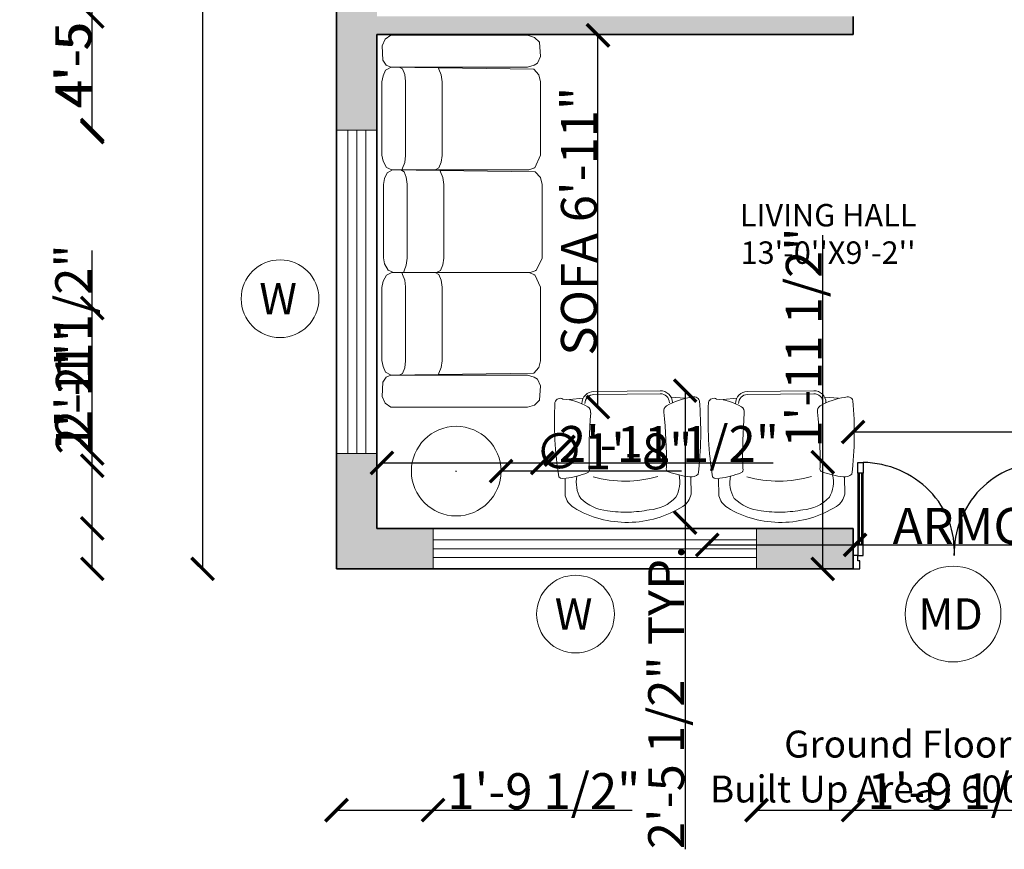
# Model space of a CAD drawing. Units: inches. Extents: x 2209 to 2954, y 1760 to 2265.
# Tile 1 of 7: x 2209 to 2428, y 1760 to 1945. Entities that reach past the tile are written whole.
import ezdxf

# ---------------------------------------------------------------- set-up
doc = ezdxf.new("R2010")
doc.units = ezdxf.units.IN
for name, color, linetype, lineweight in [('A-ANNO-DIMS', 2, 'Continuous', 18), ('A-ANNO-SYMB', 7, 'Continuous', 18), ('A-ANNO-TEXT', 7, 'Continuous', 25), ('A-AREA-IDEN', 7, 'Continuous', 18), ('A-FURN', 8, 'Continuous', 18), ('A-WALL-PATT', 30, 'Continuous', 13), ('DOOR', 240, 'Continuous', 25), ('WALL', 7, 'Continuous', 35), ('WINDOW', 190, 'Continuous', 18)]:
    doc.layers.add(name, color=color, linetype=linetype, lineweight=lineweight)
doc.layers.add('A-Glaz', color=92, linetype='Continuous')
doc.layers.add('MAIN DOOR', color=150, linetype='Continuous')
doc.styles.get("Standard").update_dxf_attribs({"font": 'arial.ttf'})
doc.dimstyles.get("Standard").update_dxf_attribs({"dimtxt": 8, "dimasz": 5, "dimexe": 0.18, "dimexo": 0.0625, "dimgap": 0.09, "dimtad": 1, "dimdec": 1, "dimzin": 0, "dimdsep": 46, "dimlunit": 4, "dimtxsty": 'Standard', "dimblk": 'ARCHTICK', "dimcen": 0.09, "dimse1": 1, "dimse2": 1, "dimadec": 0, "dimazin": 0, "dimtfac": 1, "dimtdec": 1, "dimtofl": 0, "dimtmove": 0, "dimatfit": 3, "dimfxl": 1, "dimtolj": 1, "dimtzin": 0, "dimarcsym": 0})

# ---------------------------------------------------------------- blocks, each defined once
blk = doc.blocks.new('A$C13CE0A17')
at = {"layer": 'A-Glaz'}
for p, q in [((0.01, 0.61), (0.01, 0.08)), ((0.03, 0.08), (0.03, 0.61))]:
    blk.add_line(p, q, dxfattribs=at)
blk.add_lwpolyline([(1.4, 0.08), (1.4, 0.61), (1.42, 0.61), (1.42, 0.08)], close=True, dxfattribs=at)
at = {"layer": 'MAIN DOOR'}
for p, q in [((0, 0.61), (0, 0.69)), ((0, 0.69), (0.04, 0.69)), ((0.04, 0.69), (0.04, 0.61)), ((0, 0.61), (0, 0.08)), ((0.04, 0.61), (0, 0.61)), ((0.04, 0.61), (0, 0.61)), ((0.03, 0.61), (0.01, 0.61)), ((0.04, 0.08), (0.04, 0.61)), ((0, 0.08), (0, 0)), ((0.04, 0.08), (0, 0.08)), ((0, 0.08), (0.04, 0.08)), ((0.01, 0.08), (0.03, 0.08)), ((0.04, 0), (0.04, 0.08)), ((-0.035, 0), (-0.035, -0.1)), ((0, 0), (-0.035, 0)), ((0, 0), (0.04, 0)), ((0, -0.04), (0, 0)), ((0.015, -0.04), (0, -0.04)), ((0.015, -0.05), (0.015, -0.04)), ((0.015, -0.1), (0.015, -0.05)), ((-0.035, -0.1), (0.015, -0.1))]:
    blk.add_line(p, q, dxfattribs=at)
for points in [[(1.39, 0.69), (1.39, 0.61), (1.43, 0.61), (1.43, 0.69)], [(1.39, 0.08), (1.39, 0.61), (1.43, 0.61), (1.43, 0.08)], [(1.39, 0), (1.39, 0.08), (1.43, 0.08), (1.43, 0)], [(1.43, 0), (1.465, 0), (1.465, -0.1), (1.415, -0.1), (1.415, -0.05), (1.415, -0.04), (1.43, -0.04)]]:
    blk.add_lwpolyline(points, close=True, dxfattribs=at)
blk.add_arc((1.3872, 0.017), 0.673, 89.76573, 181.44381, dxfattribs=at)
blk.add_ellipse((0.0389, 0.0511), major_axis=(0.6669, -0.1217), ratio=0.940794, start_param=0.11153, end_param=1.73917, dxfattribs=at)
blk = doc.blocks.new('12PCOU17')
at = {"color": 0, "linetype": 'ByBlock'}
for points in [[(-34.71, 34.72), (-33.66, 34.31), (-3.27, 34.3), (-1.81, 34.76), (-1.05, 35.2), (-0.38, 36.65), (-0.61, 39.84), (-1.73, 40.94), (-3.27, 41.4), (-33.66, 41.4), (-34.95, 40.5), (-35.65, 39.02), (-35.49, 35.83), (-34.71, 34.72)], [(-1.89, 11.91), (-1.66, 11.91), (-0.35, 14.68), (-0.35, 31.05), (-0.74, 32.58), (-1.89, 33.83), (-33.63, 34.3), (-34.84, 33.63), (-35.43, 32.38), (-35.68, 31), (-35.68, 14.74), (-35.43, 13.36), (-34.66, 11.99), (-33.44, 11.43), (-3, 11.44), (-1.66, 11.91)], [(-31.25, 11.43), (-31.06, 11.84), (-30.6, 13.09), (-30.4, 14.62), (-30.4, 31.12), (-30.6, 32.65), (-31.06, 33.9), (-31.81, 34.3)], [(-23.84, 11.43), (-22.99, 11.9), (-22.46, 13.15), (-22.23, 14.67), (-22.23, 31.07), (-22.46, 32.59), (-22.99, 33.84), (-23.12, 34.3)], [(-1.54, -10.96), (-1.31, -10.96), (0, -8.19), (0, 8.19), (-0.39, 9.71), (-1.54, 10.96), (-33.28, 11.44), (-34.5, 10.77), (-35.08, 9.51), (-35.33, 8.14), (-35.33, -8.13), (-35.08, -9.51), (-34.31, -10.87), (-33.1, -11.44), (-2.65, -11.43), (-1.31, -10.96)], [(-30.9, -11.44), (-30.72, -11.02), (-30.25, -9.77), (-30.05, -8.25), (-30.05, 8.26), (-30.25, 9.78), (-30.72, 11.03), (-31.47, 11.44)], [(-23.49, -11.44), (-22.64, -10.96), (-22.11, -9.72), (-21.88, -8.19), (-21.88, 8.2), (-22.11, 9.73), (-22.64, 10.97), (-22.77, 11.44)], [(-1.89, -11.91), (-1.66, -11.91), (-0.35, -14.68), (-0.35, -31.05), (-0.74, -32.58), (-1.89, -33.83), (-33.63, -34.3), (-34.84, -33.63), (-35.43, -32.38), (-35.68, -31), (-35.68, -14.74), (-35.43, -13.36), (-34.66, -11.99), (-33.44, -11.43), (-3, -11.44), (-1.66, -11.91)], [(-31.25, -11.43), (-31.06, -11.84), (-30.6, -13.09), (-30.4, -14.62), (-30.4, -31.12), (-30.6, -32.65), (-31.06, -33.9), (-31.81, -34.3)], [(-23.84, -11.43), (-22.99, -11.9), (-22.46, -13.15), (-22.23, -14.67), (-22.23, -31.07), (-22.46, -32.59), (-22.99, -33.84), (-23.12, -34.3)], [(-34.71, -34.72), (-33.66, -34.31), (-3.27, -34.3), (-1.81, -34.76), (-1.05, -35.2), (-0.38, -36.65), (-0.61, -39.84), (-1.73, -40.94), (-3.27, -41.4), (-33.66, -41.4), (-34.95, -40.5), (-35.65, -39.02), (-35.49, -35.83), (-34.71, -34.72)]]:
    blk.add_lwpolyline(points, dxfattribs=at)
blk = doc.blocks.new('A$C198557BC')
for p, q in [((-0.4117, 0.5807), (-0.4097, 0.6946)), ((0.4248, 0.5712), (0.4254, 0.6851)), ((-0.2994, 0.0834), (-0.2994, 0.0852)), ((0.3012, 0.0766), (0.3012, 0.0783)), ((-0.2905, 0.0459), (-0.3822, 0.0549)), ((0, 0), (-0.2203, 0.0025)), ((0.0002, 0.02), (-0.2201, 0.0225)), ((0, 0), (0.2203, -0.0025)), ((0.0002, 0.02), (0.2205, 0.0175)), ((0.2915, 0.0393), (0.3834, 0.0462))]:
    blk.add_line(p, q)
for centre, radius, start, end in [((-0.0029, 0.1962), 0.6755, 88.91413, 121.26982), ((0.0052, 0.1888), 0.6828, 57.60493, 89.60231), ((-0.1087, 0.5143), 0.2805, 94.11543, 135.13675), ((-0.0116, 0.1353), 0.6691, 87.97145, 100.08803), ((-0.0406, -0.2707), 1.076, 79.8996, 87.1923), ((0.1307, 0.5261), 0.2631, 42.84347, 86.21861), ((-0.2885, 0.6678), 0.1242, 121.56358, 167.53067), ((0.3036, 0.661), 0.1242, 11.16492, 57.13201), ((-0.132, 0.6064), 0.2049, 148.9368, 191.77668), ((0.1457, 0.6033), 0.2049, 346.91891, 29.75879), ((-0.0152, -0.1978), 0.7955, 73.93972, 105.23292), ((1.9871, 0.1943), 2.4688, 171.25046, 182.77379), ((-0.4204, 0.533), 0.0491, 69.35384, 131.44148), ((-0.4978, -0.067), 0.6529, 68.98758, 81.6584), ((-0.2691, 0.5224), 0.0208, 332.44605, 75.17429), ((0.2809, 0.5161), 0.0208, 103.52131, 206.24954), ((0.4962, -0.0783), 0.6529, 97.03719, 109.70801), ((0.4268, 0.5037), 0.0668, 46.11764, 99.16123), ((-1.9034, 0.2728), 2.3929, 354.99182, 6.69659), ((3.0866, 0.4124), 3.3387, 178.2785, 184.60096), ((-3.0764, 0.4826), 3.3387, 354.09463, 0.41709), ((-0.2813, 0.1392), 0.0403, 300.81783, 7.8066), ((0.2844, 0.1327), 0.0403, 170.889, 237.87776), ((-0.4437, 0.0838), 0.0362, 194.45648, 300.66989), ((-0.4522, 0.4253), 0.3736, 274.13358, 300.83861), ((-0.2194, 0.0825), 0.08, 179.3478, 269.3478), ((-0.2194, 0.0825), 0.06, 179.3478, 269.3478), ((0.2212, 0.0775), 0.08, 269.3478, 359.3478), ((0.2212, 0.0775), 0.06, 269.3478, 359.3478), ((0.4617, 0.4149), 0.3736, 237.85698, 264.56202), ((0.4455, 0.0737), 0.0362, 238.0257, 344.23911)]:
    blk.add_arc(centre, radius, start, end)
blk = doc.blocks.new('_ArchTick')
at = {"color": 0, "linetype": 'ByBlock', "const_width": 0.15}
blk.add_lwpolyline([(-0.5, -0.5), (0.5, 0.5)], dxfattribs=at)
blk = doc.blocks.new('*D14')
at = {"layer": 'A-ANNO-DIMS', "color": 0, "lineweight": -2, "transparency": 16777216}
blk.add_line((2249.34, 2182.29), (2249.34, 1822.29), dxfattribs=at)
at = {"layer": 'Defpoints', "color": 0, "transparency": 16777216}
for p in [(2279.15, 2182.29), (2249.34, 1822.29), (2279.15, 1822.29)]:
    blk.add_point(p, dxfattribs=at)
at = {"layer": 'A-ANNO-DIMS', "color": 0, "lineweight": -2, "transparency": 16777216, "xscale": 5, "yscale": 5, "zscale": 5}
for p, rotation in [((2249.34, 2182.29), 90), ((2249.34, 1822.29), 270)]:
    blk.add_blockref('_ArchTick', p, dxfattribs=dict(at, rotation=rotation))
at = {"layer": 'A-ANNO-DIMS', "color": 0, "transparency": 16777216, "insert": (2245.16, 2002.29), "char_height": 8, "attachment_point": 5, "rotation": 90}
blk.add_mtext("\\A1;30'", dxfattribs=at)
blk = doc.blocks.new('WIN-W-72IN')
for p, q in [((0, 6.5), (72, 6.5)), ((0, 4.5), (72, 4.5)), ((0, 2.5), (72, 2.5))]:
    blk.add_line(p, q)
blk.add_lwpolyline([(0, 9), (72, 9), (72, 0), (0, 0)], close=True)
blk = doc.blocks.new('TAG-OPENING-W')
blk.add_circle((0, 0), 8.66)
blk.add_text('W', height=7).set_placement((-4.62, -3.5))
blk = doc.blocks.new('*D49')
at = {"layer": 'A-ANNO-DIMS', "color": 0, "lineweight": -2, "transparency": 16777216}
for p, q in [((2394.15, 1852.78), (2439.18, 1852.78)), ((2439.18, 1852.78), (2532.94, 1852.78))]:
    blk.add_line(p, q, dxfattribs=at)
at = {"layer": 'Defpoints', "color": 0, "transparency": 16777216}
for p in [(2439.18, 1852.78), (2394.15, 1846.02), (2439.18, 1846.02)]:
    blk.add_point(p, dxfattribs=at)
at = {"layer": 'A-ANNO-DIMS', "color": 0, "lineweight": -2, "transparency": 16777216, "xscale": 5, "yscale": 5, "zscale": 5, "rotation": 180}
blk.add_blockref('_ArchTick', (2394.15, 1852.78), dxfattribs=at)
at = {"layer": 'A-ANNO-DIMS', "color": 0, "lineweight": -2, "transparency": 16777216, "xscale": 5, "yscale": 5, "zscale": 5}
blk.add_blockref('_ArchTick', (2439.18, 1852.78), dxfattribs=at)
at = {"layer": 'A-ANNO-DIMS', "color": 0, "transparency": 16777216, "insert": (2488.56, 1857.01), "char_height": 8, "attachment_point": 5}
blk.add_mtext('\\A1;MAIN DOOR 3\'-9"', dxfattribs=at)
blk = doc.blocks.new('*D50')
at = {"layer": 'A-ANNO-DIMS', "color": 0, "lineweight": -2, "transparency": 16777216}
for p, q in [((2387.4, 1846.02), (2387.4, 1896.57)), ((2387.4, 1822.29), (2387.4, 1846.02))]:
    blk.add_line(p, q, dxfattribs=at)
at = {"layer": 'Defpoints', "color": 0, "transparency": 16777216}
for p in [(2387.4, 1846.02), (2394.15, 1846.02), (2394.15, 1822.29)]:
    blk.add_point(p, dxfattribs=at)
at = {"layer": 'A-ANNO-DIMS', "color": 0, "lineweight": -2, "transparency": 16777216, "xscale": 5, "yscale": 5, "zscale": 5}
for p, rotation in [((2387.4, 1846.02), 90), ((2387.4, 1822.29), 270)]:
    blk.add_blockref('_ArchTick', p, dxfattribs=dict(at, rotation=rotation))
at = {"layer": 'A-ANNO-DIMS', "color": 0, "transparency": 16777216, "insert": (2383.17, 1873.8), "char_height": 8, "attachment_point": 5, "rotation": 90}
blk.add_mtext('\\A1;1\'-11 1/2"', dxfattribs=at)
blk = doc.blocks.new('*D59')
at = {"layer": 'A-ANNO-DIMS', "color": 0, "lineweight": -2, "transparency": 16777216}
for p, q in [((2361.69, 1827.63), (2394.59, 1827.63)), ((2394.59, 1827.63), (2511.71, 1827.63))]:
    blk.add_line(p, q, dxfattribs=at)
at = {"layer": 'Defpoints', "color": 0, "transparency": 16777216}
for p in [(2361.69, 1832.57), (2394.59, 1832.57), (2394.59, 1827.63)]:
    blk.add_point(p, dxfattribs=at)
at = {"layer": 'A-ANNO-DIMS', "color": 0, "lineweight": -2, "transparency": 16777216, "xscale": 5, "yscale": 5, "zscale": 5, "rotation": 180}
blk.add_blockref('_ArchTick', (2361.69, 1827.63), dxfattribs=at)
at = {"layer": 'A-ANNO-DIMS', "color": 0, "lineweight": -2, "transparency": 16777216, "xscale": 5, "yscale": 5, "zscale": 5}
blk.add_blockref('_ArchTick', (2394.59, 1827.63), dxfattribs=at)
at = {"layer": 'A-ANNO-DIMS', "color": 0, "transparency": 16777216, "insert": (2455.65, 1831.86), "char_height": 8, "attachment_point": 5}
blk.add_mtext('\\A1;ARMCHAIR 2\'-9" TYP.', dxfattribs=at)
blk = doc.blocks.new('*D60')
at = {"layer": 'A-ANNO-DIMS', "color": 0, "lineweight": -2, "transparency": 16777216}
for p, q in [((2356.76, 1861.96), (2356.76, 1832.57)), ((2356.76, 1832.57), (2356.76, 1759.85))]:
    blk.add_line(p, q, dxfattribs=at)
at = {"layer": 'Defpoints', "color": 0, "transparency": 16777216}
for p in [(2361.69, 1861.96), (2356.76, 1832.57), (2361.69, 1832.57)]:
    blk.add_point(p, dxfattribs=at)
at = {"layer": 'A-ANNO-DIMS', "color": 0, "lineweight": -2, "transparency": 16777216, "xscale": 5, "yscale": 5, "zscale": 5}
for p, rotation in [((2356.76, 1861.96), 90), ((2356.76, 1832.57), 270)]:
    blk.add_blockref('_ArchTick', p, dxfattribs=dict(at, rotation=rotation))
at = {"layer": 'A-ANNO-DIMS', "color": 0, "transparency": 16777216, "insert": (2352.53, 1793.71), "char_height": 8, "attachment_point": 5, "rotation": 90}
blk.add_mtext('\\A1;2\'-5 1/2" TYP.', dxfattribs=at)
blk = doc.blocks.new('*D63')
at = {"layer": 'A-ANNO-DIMS', "color": 0, "lineweight": -2, "transparency": 16777216}
blk.add_line((2337.35, 1858.3), (2337.35, 1941.1), dxfattribs=at)
at = {"layer": 'Defpoints', "color": 0, "transparency": 16777216}
for p in [(2324.93, 1941.1), (2337.35, 1941.1), (2324.93, 1858.3)]:
    blk.add_point(p, dxfattribs=at)
at = {"layer": 'A-ANNO-DIMS', "color": 0, "lineweight": -2, "transparency": 16777216, "xscale": 5, "yscale": 5, "zscale": 5}
for p, rotation in [((2337.35, 1941.1), 90), ((2337.35, 1858.3), 270)]:
    blk.add_blockref('_ArchTick', p, dxfattribs=dict(at, rotation=rotation))
at = {"layer": 'A-ANNO-DIMS', "color": 0, "transparency": 16777216, "insert": (2333.12, 1899.7), "char_height": 8, "attachment_point": 5, "rotation": 90}
blk.add_mtext('\\A1;SOFA 6\'-11"', dxfattribs=at)
blk = doc.blocks.new('*D64')
at = {"layer": 'A-ANNO-DIMS', "color": 0, "lineweight": -2, "transparency": 16777216}
for p, q in [((2289.25, 1845.88), (2324.93, 1845.88)), ((2324.93, 1845.88), (2376.37, 1845.88))]:
    blk.add_line(p, q, dxfattribs=at)
at = {"layer": 'Defpoints', "color": 0, "transparency": 16777216}
for p in [(2289.25, 1858.3), (2324.93, 1858.3), (2324.93, 1845.88)]:
    blk.add_point(p, dxfattribs=at)
at = {"layer": 'A-ANNO-DIMS', "color": 0, "lineweight": -2, "transparency": 16777216, "xscale": 5, "yscale": 5, "zscale": 5, "rotation": 180}
blk.add_blockref('_ArchTick', (2289.25, 1845.88), dxfattribs=at)
at = {"layer": 'A-ANNO-DIMS', "color": 0, "lineweight": -2, "transparency": 16777216, "xscale": 5, "yscale": 5, "zscale": 5}
blk.add_blockref('_ArchTick', (2324.93, 1845.88), dxfattribs=at)
at = {"layer": 'A-ANNO-DIMS', "color": 0, "transparency": 16777216, "insert": (2353.15, 1850.1), "char_height": 8, "attachment_point": 5}
blk.add_mtext('\\A1;2\'-11 1/2"', dxfattribs=at)
blk = doc.blocks.new('*D68')
at = {"layer": 'A-ANNO-DIMS', "color": 0, "lineweight": -2, "transparency": 16777216}
for p, q in [((2279.15, 1768.57), (2300.65, 1768.57)), ((2300.65, 1768.57), (2344.99, 1768.57))]:
    blk.add_line(p, q, dxfattribs=at)
at = {"layer": 'Defpoints', "color": 0, "transparency": 16777216}
for p in [(2279.15, 1822.29), (2300.65, 1822.29), (2300.65, 1768.57)]:
    blk.add_point(p, dxfattribs=at)
at = {"layer": 'A-ANNO-DIMS', "color": 0, "lineweight": -2, "transparency": 16777216, "xscale": 5, "yscale": 5, "zscale": 5, "rotation": 180}
blk.add_blockref('_ArchTick', (2279.15, 1768.57), dxfattribs=at)
at = {"layer": 'A-ANNO-DIMS', "color": 0, "lineweight": -2, "transparency": 16777216, "xscale": 5, "yscale": 5, "zscale": 5}
blk.add_blockref('_ArchTick', (2300.65, 1768.57), dxfattribs=at)
at = {"layer": 'A-ANNO-DIMS', "color": 0, "transparency": 16777216, "insert": (2325.32, 1772.79), "char_height": 8, "attachment_point": 5}
blk.add_mtext('\\A1;1\'-9 1/2"', dxfattribs=at)
blk = doc.blocks.new('*D69')
at = {"layer": 'A-ANNO-DIMS', "color": 0, "lineweight": -2, "transparency": 16777216}
for p, q in [((2372.65, 1768.57), (2394.15, 1768.57)), ((2394.15, 1768.57), (2438.49, 1768.57))]:
    blk.add_line(p, q, dxfattribs=at)
at = {"layer": 'Defpoints', "color": 0, "transparency": 16777216}
for p in [(2372.65, 1822.29), (2394.15, 1822.29), (2394.15, 1768.57)]:
    blk.add_point(p, dxfattribs=at)
at = {"layer": 'A-ANNO-DIMS', "color": 0, "lineweight": -2, "transparency": 16777216, "xscale": 5, "yscale": 5, "zscale": 5, "rotation": 180}
blk.add_blockref('_ArchTick', (2372.65, 1768.57), dxfattribs=at)
at = {"layer": 'A-ANNO-DIMS', "color": 0, "lineweight": -2, "transparency": 16777216, "xscale": 5, "yscale": 5, "zscale": 5}
blk.add_blockref('_ArchTick', (2394.15, 1768.57), dxfattribs=at)
at = {"layer": 'A-ANNO-DIMS', "color": 0, "transparency": 16777216, "insert": (2418.82, 1772.79), "char_height": 8, "attachment_point": 5}
blk.add_mtext('\\A1;1\'-9 1/2"', dxfattribs=at)
blk = doc.blocks.new('*D71')
at = {"layer": 'A-ANNO-DIMS', "color": 0, "lineweight": -2, "transparency": 16777216}
for p, q in [((2224.78, 1847.97), (2224.78, 1893.19)), ((2224.78, 1822.29), (2224.78, 1847.97))]:
    blk.add_line(p, q, dxfattribs=at)
at = {"layer": 'Defpoints', "color": 0, "transparency": 16777216}
for p in [(2224.78, 1847.97), (2279.15, 1847.97), (2279.15, 1822.29)]:
    blk.add_point(p, dxfattribs=at)
at = {"layer": 'A-ANNO-DIMS', "color": 0, "lineweight": -2, "transparency": 16777216, "xscale": 5, "yscale": 5, "zscale": 5}
for p, rotation in [((2224.78, 1847.97), 90), ((2224.78, 1822.29), 270)]:
    blk.add_blockref('_ArchTick', p, dxfattribs=dict(at, rotation=rotation))
at = {"layer": 'A-ANNO-DIMS', "color": 0, "transparency": 16777216, "insert": (2220.55, 1873.08), "char_height": 8, "attachment_point": 5, "rotation": 90}
blk.add_mtext('\\A1;2\'-1 1/2"', dxfattribs=at)
blk = doc.blocks.new('*D72')
at = {"layer": 'A-ANNO-DIMS', "color": 0, "lineweight": -2, "transparency": 16777216}
blk.add_line((2224.78, 1919.97), (2224.78, 1973.29), dxfattribs=at)
at = {"layer": 'Defpoints', "color": 0, "transparency": 16777216}
for p in [(2224.78, 1973.29), (2279.15, 1973.29), (2279.15, 1919.97)]:
    blk.add_point(p, dxfattribs=at)
at = {"layer": 'A-ANNO-DIMS', "color": 0, "lineweight": -2, "transparency": 16777216, "xscale": 5, "yscale": 5, "zscale": 5}
for p, rotation in [((2224.78, 1973.29), 90), ((2224.78, 1919.97), 270)]:
    blk.add_blockref('_ArchTick', p, dxfattribs=dict(at, rotation=rotation))
at = {"layer": 'A-ANNO-DIMS', "color": 0, "transparency": 16777216, "insert": (2220.55, 1946.63), "char_height": 8, "attachment_point": 5, "rotation": 90}
blk.add_mtext('\\A1;4\'-5 1/2"', dxfattribs=at)
blk = doc.blocks.new('*D78')
at = {"layer": 'A-ANNO-DIMS', "color": 0, "lineweight": -2, "transparency": 16777216}
blk.add_line((2224.78, 1945.29), (2224.78, 1981.29), dxfattribs=at)
at = {"layer": 'Defpoints', "color": 0, "transparency": 16777216}
for p in [(2224.78, 1981.29), (2288.15, 1981.29), (2288.15, 1945.29)]:
    blk.add_point(p, dxfattribs=at)
at = {"layer": 'A-ANNO-DIMS', "color": 0, "lineweight": -2, "transparency": 16777216, "xscale": 5, "yscale": 5, "zscale": 5}
for p, rotation in [((2224.78, 1981.29), 90), ((2224.78, 1945.29), 270)]:
    blk.add_blockref('_ArchTick', p, dxfattribs=dict(at, rotation=rotation))
at = {"layer": 'A-ANNO-DIMS', "color": 0, "transparency": 16777216, "insert": (2220.6, 1963.29), "char_height": 8, "attachment_point": 5, "rotation": 90}
blk.add_mtext('\\A1;3\'-0"', dxfattribs=at)
blk = doc.blocks.new('*D83')
at = {"layer": 'A-ANNO-DIMS', "color": 0, "lineweight": -2, "transparency": 16777216}
blk.add_line((2224.78, 1845.25), (2224.78, 1880.36), dxfattribs=at)
at = {"layer": 'Defpoints', "color": 0, "transparency": 16777216}
for p in [(2224.78, 1880.36), (2489.03, 1880.36), (2489.03, 1845.25)]:
    blk.add_point(p, dxfattribs=at)
at = {"layer": 'A-ANNO-DIMS', "color": 0, "lineweight": -2, "transparency": 16777216, "xscale": 5, "yscale": 5, "zscale": 5}
for p, rotation in [((2224.78, 1880.36), 90), ((2224.78, 1845.25), 270)]:
    blk.add_blockref('_ArchTick', p, dxfattribs=dict(at, rotation=rotation))
at = {"layer": 'A-ANNO-DIMS', "color": 0, "transparency": 16777216, "insert": (2220.67, 1862.81), "char_height": 8, "attachment_point": 5, "rotation": 90}
blk.add_mtext('\\A1;2\'-11"', dxfattribs=at)
blk = doc.blocks.new('*D84')
at = {"layer": 'A-ANNO-DIMS', "color": 0, "lineweight": -2, "transparency": 16777216}
for p, q in [((2224.78, 1845.25), (2224.78, 1870.94)), ((2224.78, 1831.29), (2224.78, 1845.25))]:
    blk.add_line(p, q, dxfattribs=at)
at = {"layer": 'Defpoints', "color": 0, "transparency": 16777216}
for p in [(2224.78, 1845.25), (2489.03, 1845.25), (2486.15, 1831.29)]:
    blk.add_point(p, dxfattribs=at)
at = {"layer": 'A-ANNO-DIMS', "color": 0, "lineweight": -2, "transparency": 16777216, "xscale": 5, "yscale": 5, "zscale": 5}
for p, rotation in [((2224.78, 1845.25), 90), ((2224.78, 1831.29), 270)]:
    blk.add_blockref('_ArchTick', p, dxfattribs=dict(at, rotation=rotation))
at = {"layer": 'A-ANNO-DIMS', "color": 0, "transparency": 16777216, "insert": (2220.67, 1860.6), "char_height": 8, "attachment_point": 5, "rotation": 90}
blk.add_mtext('\\A1;1\'-2"', dxfattribs=at)
blk = doc.blocks.new('*D88')
at = {"layer": 'A-ANNO-DIMS', "color": 0, "lineweight": -2, "transparency": 16777216}
blk.add_line((2224.78, 1919.53), (2224.78, 1973.14), dxfattribs=at)
at = {"layer": 'Defpoints', "color": 0, "transparency": 16777216}
for p in [(2224.78, 1973.14), (2629.22, 1973.14), (2629.22, 1919.53)]:
    blk.add_point(p, dxfattribs=at)
at = {"layer": 'A-ANNO-DIMS', "color": 0, "lineweight": -2, "transparency": 16777216, "xscale": 5, "yscale": 5, "zscale": 5}
for p, rotation in [((2224.78, 1973.14), 90), ((2224.78, 1919.53), 270)]:
    blk.add_blockref('_ArchTick', p, dxfattribs=dict(at, rotation=rotation))
at = {"layer": 'A-ANNO-DIMS', "color": 0, "transparency": 16777216, "insert": (2220.55, 1946.34), "char_height": 8, "attachment_point": 5, "rotation": 90}
blk.add_mtext('\\A1;4\'-5 1/2"', dxfattribs=at)
blk = doc.blocks.new('*D94')
at = {"layer": 'A-ANNO-DIMS', "color": 0, "lineweight": -2, "transparency": 16777216}
for p, q in [((2305.71, 1844.05), (2305.89, 1844.05)), ((2305.8, 1843.96), (2305.8, 1844.14)), ((2355.94, 1844.05), (2315.79, 1844.05))]:
    blk.add_line(p, q, dxfattribs=at)
at = {"layer": 'Defpoints', "color": 0, "transparency": 16777216}
for p in [(2295.82, 1844.05), (2315.79, 1844.05)]:
    blk.add_point(p, dxfattribs=at)
at = {"layer": 'A-ANNO-DIMS', "color": 0, "lineweight": -2, "transparency": 16777216, "xscale": 5, "yscale": 5, "zscale": 5, "rotation": 179.9972683628424}
blk.add_blockref('_ArchTick', (2315.79, 1844.05), dxfattribs=at)
at = {"layer": 'A-ANNO-DIMS', "color": 0, "transparency": 16777216, "insert": (2340.86, 1848.45), "char_height": 8, "attachment_point": 5, "rotation": 359.9973}
blk.add_mtext('\\A1;∅1\'-8"', dxfattribs=at)

msp = doc.modelspace()

# ---------------------------------------------------------------- hatches: boundary and pattern name
at = {"layer": 'A-WALL-PATT', "transparency": 33554585}
h = msp.add_hatch(color=256, dxfattribs=at)
h.dxf.hatch_style = 1
h.paths.add_polyline_path([(2519.15, 2182.29), (2402.15, 2182.29), (2402.15, 2173.29), (2444.15, 2173.29), (2444.15, 2154.12), (2448.15, 2154.12), (2448.15, 2173.29), (2510.15, 2173.29), (2510.15, 2167.29), (2519.15, 2167.29)])
h.paths.add_polyline_path([(2330.15, 2182.29), (2279.15, 2182.29), (2279.15, 2145.83), (2288.15, 2145.83), (2288.15, 2158.01), (2288.15, 2173.29), (2330.15, 2173.29)])
h.paths.add_polyline_path([(2288.15, 2073.83), (2279.15, 2073.83), (2279.15, 2009.29), (2288.15, 2009.29), (2288.15, 2037.29), (2404.15, 2037.29), (2404.15, 2041.29), (2288.15, 2041.29)])
h.paths.add_polyline_path([(2519.15, 2131.29), (2510.15, 2131.29), (2510.15, 2125.29), (2444.15, 2125.29), (2444.15, 2041.29), (2439.11, 2041.29), (2439.11, 2037.29), (2448.15, 2037.29), (2448.15, 2069.29), (2481.65, 2069.29), (2481.65, 2073.29), (2448.15, 2073.29), (2448.15, 2121.29), (2468.19, 2121.29), (2468.19, 2121.32), (2488.37, 2121.32), (2510.15, 2121.29), (2510.15, 2113.63), (2519.15, 2113.63)])
h.paths.add_polyline_path([(2519.15, 2077.63), (2510.15, 2077.63), (2510.15, 2073.32), (2510.17, 2073.32), (2510.15, 2069.19), (2510.15, 2043.25), (2519.15, 2043.25)], flags=17)
h.paths.add_polyline_path([(2519.15, 1971.25), (2510.15, 1971.25), (2510.15, 1945.29), (2444.15, 1945.29), (2444.15, 1937.21), (2448.15, 1937.21), (2448.15, 1941.29), (2510.15, 1941.29), (2510.15, 1922.29), (2519.15, 1922.29)])
h.paths.add_polyline_path([(2288.15, 1941.29), (2394.15, 1941.29), (2394.15, 1945.29), (2288.15, 1945.29), (2288.15, 1973.29), (2279.15, 1973.29), (2279.15, 1919.97), (2288.15, 1919.97)])
h.paths.add_polyline_path([(2300.65, 1831.29), (2288.15, 1831.29), (2288.15, 1847.97), (2279.15, 1847.97), (2279.15, 1822.29), (2300.65, 1822.29)])
h.paths.add_polyline_path([(2394.15, 1825.29), (2394.15, 1831.29), (2372.65, 1831.29), (2372.65, 1822.29), (2394.15, 1822.29)])
h.paths.add_polyline_path([(2449.17, 1831.29), (2448.15, 1831.29), (2448.15, 1899.32), (2444.15, 1899.32), (2444.15, 1831.29), (2439.18, 1831.29), (2439.18, 1822.29), (2449.17, 1822.29)])
h.paths.add_polyline_path([(2519.15, 1850.29), (2510.15, 1850.29), (2510.15, 1831.29), (2509.17, 1831.29), (2509.17, 1822.29), (2519.15, 1822.29)])
h.paths.add_polyline_path([(2638.22, 1941.29), (2744.22, 1941.29), (2744.22, 1945.29), (2638.22, 1945.29), (2638.22, 1973.14), (2629.22, 1973.14), (2629.22, 1919.53), (2638.22, 1919.53)])
h.paths.add_polyline_path([(2638.22, 1847.53), (2629.22, 1847.53), (2629.22, 1822.29), (2650.72, 1822.29), (2650.72, 1831.29), (2638.22, 1831.29)])
h.paths.add_polyline_path([(2638.22, 2037.29), (2754.22, 2037.29), (2754.22, 2041.29), (2638.22, 2041.29), (2638.22, 2074.27), (2629.22, 2074.27), (2629.22, 2009.14), (2638.22, 2009.14)])
h.paths.add_polyline_path([(2803.22, 1936.29), (2812.78, 1936.29), (2812.78, 1945.29), (2791.22, 1945.29), (2791.22, 1936.29), (2794.22, 1936.29), (2794.22, 1831.29), (2722.72, 1831.29), (2722.72, 1822.29), (2803.22, 1822.29)])
h.paths.add_polyline_path([(2869.22, 1955.43), (2860.22, 1955.43), (2860.22, 1945.29), (2853.36, 1945.29), (2853.36, 1936.29), (2869.22, 1936.29)])
h.paths.add_polyline_path([(2680.22, 2182.29), (2629.22, 2182.29), (2629.22, 2146.27), (2638.22, 2146.27), (2638.22, 2173.29), (2680.22, 2173.29)])
h.paths.add_polyline_path([(2869.22, 2182.29), (2752.22, 2182.29), (2752.22, 2173.29), (2794.22, 2173.29), (2794.22, 2142.92), (2798.22, 2142.92), (2798.22, 2173.29), (2860.22, 2173.29), (2860.22, 2158.46), (2869.22, 2158.46)])
h.paths.add_polyline_path([(2869.22, 2122.46), (2860.22, 2122.46), (2860.22, 2090.29), (2869.22, 2090.29)])

# ---------------------------------------------------------------- linework, layer by layer
at = {"layer": 'A-ANNO-SYMB'}
msp.add_circle((2416.4, 1812.24), 10.67, dxfattribs=at)
at = {"layer": 'A-FURN'}
msp.add_circle((2305.8, 1844.05), 9.98, dxfattribs=at)
at = {"layer": 'WALL'}
for p, q in [((2279.15, 2182.29), (2279.15, 1822.29)), ((2394.15, 1945.29), (2394.15, 1941.29)), ((2288.15, 1941.29), (2394.15, 1941.29)), ((2288.15, 1941.29), (2288.15, 1831.29)), ((2288.15, 1831.29), (2394.15, 1831.29)), ((2394.15, 1831.29), (2394.15, 1822.29)), ((2279.15, 1822.29), (2394.15, 1822.29))]:
    msp.add_line(p, q, dxfattribs=at)

# ---------------------------------------------------------------- block references
at = {"layer": 'A-ANNO-SYMB'}
for p in [(2266.58, 1882.44), (2332.36, 1812.22)]:
    msp.add_blockref('TAG-OPENING-W', p, dxfattribs=at)
at = {"layer": 'A-FURN'}
msp.add_blockref('12PCOU17', (2324.93, 1899.7), dxfattribs=at)
at = {"layer": 'A-FURN', "xscale": -33.52556732039916, "yscale": 33.52556732039916, "zscale": 33.52556732039916, "rotation": 180}
for p in [(2343.82, 1861.87), (2378.01, 1861.87)]:
    msp.add_blockref('A$C198557BC', p, dxfattribs=at)
at = {"layer": 'DOOR', "xscale": 30.0188950098318, "yscale": 30.0188950098318, "zscale": 30.0188950098318}
msp.add_blockref('A$C13CE0A17', (2395.21, 1825.29), dxfattribs=at)
at = {"layer": 'WINDOW', "rotation": 89.99999999999972}
msp.add_blockref('WIN-W-72IN', (2288.15, 1847.97), dxfattribs=at)
at = {"layer": 'WINDOW'}
msp.add_blockref('WIN-W-72IN', (2300.65, 1822.29), dxfattribs=at)

# ---------------------------------------------------------------- texts
at = {"layer": 'A-ANNO-SYMB'}
msp.add_text('MD', height=7, dxfattribs=at).set_placement((2408.69, 1808.74))
at = {"layer": 'A-ANNO-TEXT', "insert": (2338.03, 1786.28), "char_height": 6, "attachment_point": 1}
msp.add_mtext_dynamic_manual_height_columns('\\pxqc;Ground Floor Plan\\PBuilt Up Area : 600.00 Sq. ft', width=151.0778, gutter_width=102.73, heights=[0], dxfattribs=at)
at = {"layer": 'A-AREA-IDEN', "insert": (2366.02, 1903.54), "char_height": 5, "attachment_point": 1}
msp.add_mtext_dynamic_manual_height_columns("\\pxqc;LIVING HALL\\P13'-0''X9'-2''", width=45.1409, gutter_width=12.5, heights=[0], dxfattribs=at)

# ---------------------------------------------------------------- dimensions: what is measured, and where the dimension line sits
at = {"layer": 'A-ANNO-DIMS'}
for base, p1, p2, override, picture, middle in [((2249.34, 1822.29), (2279.15, 2182.29), (2279.15, 1822.29), {"dimclrd": 0, "dimclre": 0, "dimclrt": 0}, '*D14', (2245.16, 2002.29)), ((2224.78, 1981.29), (2288.15, 1945.29), (2288.15, 1981.29), {"dimdec": 1, "dimlfac": 1, "dimrnd": 0, "dimzin": 1, "dimdsep": 46, "dimlunit": 4, "dimfrac": 2}, '*D78', (2220.6, 1963.29)), ((2224.78, 1973.29), (2279.15, 1919.97), (2279.15, 1973.29), {"dimdec": 1, "dimlfac": 1, "dimrnd": 0, "dimzin": 1, "dimdsep": 46, "dimlunit": 4, "dimfrac": 2}, '*D72', (2220.55, 1946.63)), ((2224.78, 1973.14), (2629.22, 1919.53), (2629.22, 1973.14), {"dimdec": 1, "dimlfac": 1, "dimrnd": 0, "dimzin": 1, "dimdsep": 46, "dimlunit": 4, "dimfrac": 2}, '*D88', (2220.55, 1946.34)), ((2387.4, 1846.02), (2394.15, 1822.29), (2394.15, 1846.02), {"dimdec": 1, "dimlfac": 1, "dimrnd": 0, "dimzin": 1, "dimdsep": 46, "dimlunit": 4, "dimfrac": 2}, '*D50', (2383.17, 1873.8)), ((2224.78, 1847.97), (2279.15, 1822.29), (2279.15, 1847.97), {"dimdec": 1, "dimlfac": 1, "dimrnd": 0, "dimzin": 1, "dimdsep": 46, "dimlunit": 4, "dimfrac": 2}, '*D71', (2220.55, 1873.08)), ((2224.78, 1880.36), (2489.03, 1845.25), (2489.03, 1880.36), {"dimdec": 1, "dimlfac": 1, "dimrnd": 0, "dimzin": 1, "dimdsep": 46, "dimlunit": 4, "dimfrac": 2}, '*D83', (2220.67, 1862.81)), ((2224.78, 1845.25), (2486.15, 1831.29), (2489.03, 1845.25), {"dimdec": 1, "dimlfac": 1, "dimrnd": 0, "dimzin": 1, "dimdsep": 46, "dimlunit": 4, "dimfrac": 2}, '*D84', (2220.67, 1860.6))]:
    dim = msp.add_linear_dim(base=base, p1=p1, p2=p2, angle=90, dimstyle='Standard', override=override, dxfattribs=at)
    dim.commit()
    dim.dimension.update_dxf_attribs({"geometry": picture, "text_midpoint": middle})
for base, p1, p2, angle, text, picture, middle in [((2337.35, 1941.1), (2324.93, 1858.3), (2324.93, 1941.1), 90, 'SOFA <>', '*D63', (2333.12, 1899.7)), ((2356.76, 1832.57), (2361.69, 1861.96), (2361.69, 1832.57), 270, '<> TYP.', '*D60', (2352.53, 1793.71))]:
    dim = msp.add_linear_dim(base=base, p1=p1, p2=p2, angle=angle, text=text, dimstyle='Standard', override={"dimdec": 1, "dimlfac": 1, "dimrnd": 0, "dimzin": 1, "dimdsep": 46, "dimlunit": 4, "dimfrac": 2}, dxfattribs=at)
    dim.commit()
    dim.dimension.update_dxf_attribs({"geometry": picture, "text_midpoint": middle})
for base, p1, p2, text, picture, middle in [((2439.18, 1852.78), (2394.15, 1846.02), (2439.18, 1846.02), 'MAIN DOOR <>', '*D49', (2488.56, 1857.01)), ((2394.59, 1827.63), (2361.69, 1832.57), (2394.59, 1832.57), 'ARMCHAIR <> TYP.', '*D59', (2455.65, 1831.86))]:
    dim = msp.add_linear_dim(base=base, p1=p1, p2=p2, text=text, dimstyle='Standard', override={"dimdec": 1, "dimlfac": 1, "dimrnd": 0, "dimzin": 1, "dimdsep": 46, "dimlunit": 4, "dimfrac": 2}, dxfattribs=at)
    dim.commit()
    dim.dimension.update_dxf_attribs({"geometry": picture, "text_midpoint": middle})
for base, p1, p2, picture, middle in [((2324.93, 1845.88), (2289.25, 1858.3), (2324.93, 1858.3), '*D64', (2353.15, 1850.1)), ((2300.65, 1768.57), (2279.15, 1822.29), (2300.65, 1822.29), '*D68', (2325.32, 1772.79)), ((2394.15, 1768.57), (2372.65, 1822.29), (2394.15, 1822.29), '*D69', (2418.82, 1772.79))]:
    dim = msp.add_linear_dim(base=base, p1=p1, p2=p2, dimstyle='Standard', override={"dimdec": 1, "dimlfac": 1, "dimrnd": 0, "dimzin": 1, "dimdsep": 46, "dimlunit": 4, "dimfrac": 2}, dxfattribs=at)
    dim.commit()
    dim.dimension.update_dxf_attribs({"geometry": picture, "text_midpoint": middle})
dim = msp.add_diameter_dim_2p(p1=(2295.82, 1844.05), p2=(2315.79, 1844.05), dimstyle='Standard', override={"dimdec": 1, "dimlfac": 1, "dimrnd": 0, "dimzin": 1, "dimdsep": 46, "dimlunit": 4, "dimfrac": 2}, dxfattribs=at)
dim.commit()
dim.dimension.update_dxf_attribs({"geometry": '*D94', "text_midpoint": (2340.86, 1844.05), "dimtype": 163})

doc.saveas('drawing.dxf')
